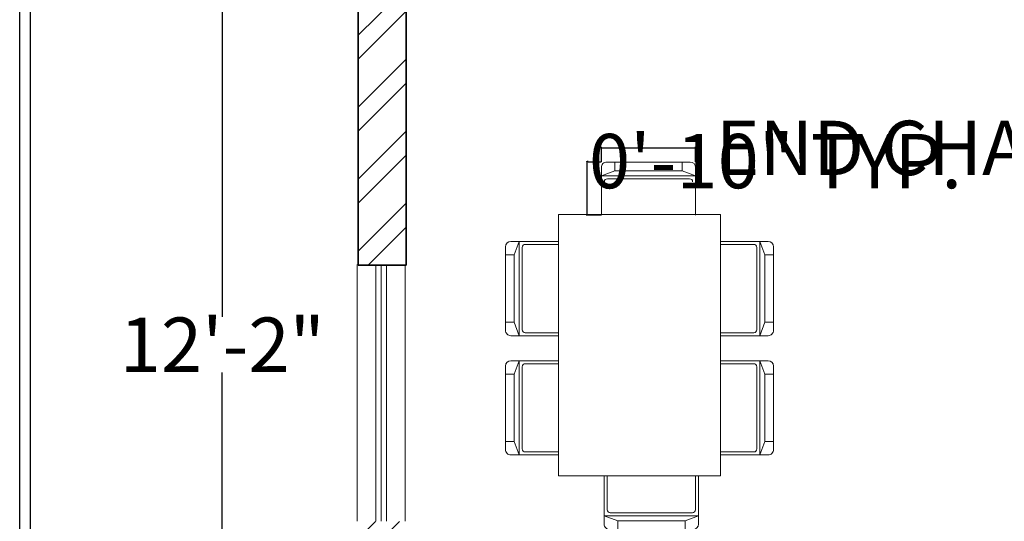
# Model space of a CAD drawing. Units: inches. Extents: x 1812 to 2791, y 2306 to 2959.
# Tile 6 of 8: x 2391 to 2575, y 2655 to 2748. Entities that reach past the tile are written whole.
import ezdxf

# ---------------------------------------------------------------- set-up
doc = ezdxf.new("R2010")
doc.units = ezdxf.units.IN
doc.layers.get('Defpoints').update_dxf_attribs({"lineweight": 50})
for name, color, linetype, lineweight in [('00 FURNITURE', 15, 'Continuous', 15), ('A-ANNO-DIMS', 2, 'Continuous', 18), ('A-ANNO-TTLB', 7, 'Continuous', 25), ('A-WALL-PATT', 8, 'Continuous', 13), ('WALL', 7, 'Continuous', 35), ('WINDOWS', 160, 'Continuous', 18)]:
    doc.layers.add(name, color=color, linetype=linetype, lineweight=lineweight)
doc.styles.get("Standard").update_dxf_attribs({"font": 'arial.ttf'})
doc.dimstyles.get("Standard").update_dxf_attribs({"dimtxt": 10.18, "dimasz": 0.18, "dimexe": 0.18, "dimexo": 0.0625, "dimgap": 0.09, "dimtad": 0, "dimtih": 1, "dimtoh": 1, "dimdec": 0, "dimzin": 0, "dimdsep": 46, "dimlunit": 3, "dimtxsty": 'Standard', "dimcen": 0.09, "dimadec": 0, "dimazin": 0, "dimtfac": 1, "dimtdec": 0, "dimtofl": 0, "dimtmove": 0, "dimatfit": 3, "dimfxl": 1, "dimtolj": 1, "dimtzin": 0, "dimarcsym": 0})

# ---------------------------------------------------------------- blocks, each defined once
blk = doc.blocks.new('CHAIR-DINING')
for p, q in [((-0.0002919860735346, 16.63588649700705), (-0.0003138742495139, 1.018845651208721)), ((9.925763979173098, 17.65493302806589), (1.018765697107482, 17.65494176689844)), ((1.614874244286511, 15.12954713197268), (2.568532326808963, 17.65494024488453)), ((2.568532326808963, 17.65494024488453), (2.568507595072333, -0.0002145154603568)), ((9.925763979173098, 17.09119695253048), (3.692750862651337, 17.09120477086708)), ((1.614874244286511, 15.12954713197268), (1.614856157536451, 2.551355148459151)), ((3.132268951824698, 16.530724333742), (3.132247167491186, 1.124003998030275)), ((1.614856157536451, 2.551355148459151), (2.568507595072333, -0.0002145154603568)), ((3.692727608225141, 0.5635220945378024), (9.925763979173098, 0.5635142763176191)), ((1.018741536737252, -0.0002124476914105), (9.925763979173098, -0.0002237815378976))]:
    blk.add_line(p, q)
blk.add_lwpolyline([(-0.000293857100587, 15.12954925550457), (-0.000311951301228, 2.551357264540456), (1.614856157536451, 2.551355148459151), (1.614874244286511, 15.12954713197268)], close=True)
for centre, radius, start, end in [((1.018764709439892, 16.63588507511031), 1.019056690993971, 89.9999438110219, 179.9999196585658), ((3.692750135055575, 16.53072360987153), 0.5604811800496505, 89.99992486791913, 179.9999248879294), ((1.018742821263913, 1.018844240487851), 1.019056690993971, 179.9999201921744, 269.9999275359618), ((3.692728335820902, 1.124003270434513), 0.5604811800496505, 179.9999248879294, 269.9999248679191)]:
    blk.add_arc(centre, radius, start, end)
blk = doc.blocks.new('CHAIR-DINING-END')
for p, q in [((16.63624727438082, 9.925777952737917), (1.019206428582492, 9.925799840913896)), ((0.0001483296823608, 8.9067444296943), (0.0001369958358737, -0.0002780127415463)), ((2.551715925832922, 8.3106298088951), (0.0001462619134145, 7.356978371592049)), ((15.12990790946287, 8.31061172214504), (2.551715925832922, 8.3106298088951)), ((15.12990790946287, 8.31061172214504), (17.6553010222583, 7.356953639622588)), ((17.65529380532325, -0.0002780127415463), (17.65530254427222, 8.9067202695569)), ((17.6553010222583, 7.356953639622588), (0.0001462619134145, 7.356978371592049)), ((16.53108511111577, 6.793217014839683), (1.124364775520461, 6.793238799173195))]:
    blk.add_line(p, q)
blk.add_lwpolyline([(15.12991003287834, 9.92577982376497), (2.551718041914227, 9.92579791773278), (2.551715925832922, 8.3106298088951), (15.12990790946287, 8.31061172214504)], close=True)
for centre, radius, start, end in [((1.019205017861622, 8.906743145400469), 1.019056690993971, 89.99992015882385, 179.9999275359617), ((16.63624585248408, 8.90672125699166), 1.019056690993971, 359.9999438110219, 89.99991962521533), ((1.124364047808285, 6.232757630610649), 0.5604811800496505, 89.99992490793976, 179.9999248679191), ((16.5310843872453, 6.232735831608806), 0.5604811800496505, 359.9999248679191, 89.99992490793976)]:
    blk.add_arc(centre, radius, start, end)
blk = doc.blocks.new('TABLE-DINING-RECT')
for p, q in [((30.34839303535387, 48.92733218540207), (-0.0002364942340591, 48.92732934110473)), ((-0.0002326415853986, 48.92732934110473), (-0.0002280560938743, 0.0001748373420014)), ((30.34839189378522, 48.92733218540207), (30.34839647927674, 0.0001776816393431)), ((30.34839647927674, 0.0001776816393431), (-0.0002280560934196, 0.0001748373420014))]:
    blk.add_line(p, q)
blk = doc.blocks.new('WINDOW-48x9')
for p, q in [((-0.0002644799014888, 47.99951726123345), (-0.0002644799014888, -0.00048273876655)), ((3.499735520098511, -0.00048273876655), (3.499735520098511, 47.99951726123345)), ((4.499735520098511, -0.00048273876655), (4.499735520098511, 47.99951726123345)), ((5.499735520098511, -0.00048273876655), (5.499735520098511, 47.99951726123345)), ((8.999735520098511, -0.00048273876655), (8.999735520098511, 47.99951726123345))]:
    blk.add_line(p, q)
blk = doc.blocks.new('SHEET-FRAME-RESIDENCE')
blk.add_lwpolyline([(0.000131823559741, 632.8005012919775), (378.7609620870107, 632.8005012919775), (378.7609620870107, 0.0003856501880364), (0.000131823559741, 0.0003856501880364)], close=True)
blk.add_lwpolyline([(2.00013182355974, 71.32450104412055), (2.00013182355974, 630.8005012919775), (376.7609620870107, 630.8005012919775), (376.7609620870107, 71.32450104412055)])
blk = doc.blocks.new('*D64')
at = {"layer": 'A-ANNO-DIMS', "color": 0, "lineweight": -2, "transparency": 16777216}
for p, q in [((2499.736887761388, 2721.901978502181), (2499.736887761388, 2724.667753417118)), ((2499.916887761388, 2724.487753417118), (2517.212053860968, 2724.487753417118)), ((2517.392053860968, 2721.901978502181), (2517.392053860968, 2724.667753417118)), ((2517.392053860968, 2724.487753417118), (2517.572053860968, 2724.487753417118))]:
    blk.add_line(p, q, dxfattribs=at)
at = {"layer": 'A-ANNO-DIMS', "color": 0, "transparency": 16777216}
for points in [[(2499.916887761388, 2724.517753417118), (2499.916887761388, 2724.457753417118), (2499.736887761388, 2724.487753417118)], [(2517.212053860968, 2724.517753417118), (2517.212053860968, 2724.457753417118), (2517.392053860968, 2724.487753417118)]]:
    blk.add_solid(points, dxfattribs=at)
at = {"layer": 'Defpoints', "color": 0, "transparency": 16777216}
for p in [(2517.392053860968, 2724.487753417118), (2499.736887761388, 2721.839478502181), (2517.392053860968, 2721.839478502181)]:
    blk.add_point(p, dxfattribs=at)
at = {"layer": 'A-ANNO-DIMS', "color": 0, "transparency": 16777216, "insert": (2601.369291241595, 2724.487753417118), "char_height": 10.18, "attachment_point": 5}
blk.add_mtext('\\A1;END CHAIR 1\'-5 1/2" TYP.', dxfattribs=at)
blk = doc.blocks.new('*D65')
at = {"layer": 'A-ANNO-DIMS', "color": 0, "lineweight": -2, "transparency": 16777216}
for p, q in [((2499.674387761389, 2721.839478502182), (2496.908612846453, 2721.839478502182)), ((2497.088612846453, 2721.839478502182), (2497.088612846453, 2722.019478502182)), ((2497.088612846453, 2722.019478502182), (2497.268612846453, 2722.019478502182)), ((2497.088612846453, 2712.093400276427), (2497.088612846453, 2721.659478502183)), ((2499.674387761389, 2711.913400276428), (2496.908612846453, 2711.913400276428))]:
    blk.add_line(p, q, dxfattribs=at)
at = {"layer": 'A-ANNO-DIMS', "color": 0, "transparency": 16777216}
for points in [[(2497.058612846453, 2721.659478502183), (2497.118612846453, 2721.659478502183), (2497.088612846453, 2721.839478502182)], [(2497.058612846453, 2712.093400276427), (2497.118612846453, 2712.093400276427), (2497.088612846453, 2711.913400276428)]]:
    blk.add_solid(points, dxfattribs=at)
at = {"layer": 'Defpoints', "color": 0, "transparency": 16777216}
for p in [(2497.088612846453, 2721.839478502182), (2499.736887761389, 2721.839478502182), (2499.736887761389, 2711.913400276428)]:
    blk.add_point(p, dxfattribs=at)
at = {"layer": 'A-ANNO-DIMS', "color": 0, "transparency": 16777216, "insert": (2532.33934272367, 2722.019478502181), "char_height": 10.18, "attachment_point": 5}
blk.add_mtext('\\A1;0\'-10" TYP.', dxfattribs=at)
blk = doc.blocks.new('*D73')
at = {"layer": 'A-ANNO-DIMS', "color": 0, "lineweight": -2, "transparency": 16777216}
for p, q in [((2454.218562000001, 2760.694666000001), (2428.586486000002, 2760.694666000001)), ((2428.766486000002, 2760.514666000001), (2428.766486000002, 2692.848797196454)), ((2428.766486000002, 2614.781264000001), (2428.766486000002, 2682.447132803548)), ((2454.176191000001, 2614.601264000001), (2428.586486000002, 2614.601264000001))]:
    blk.add_line(p, q, dxfattribs=at)
at = {"layer": 'A-ANNO-DIMS', "color": 0, "transparency": 16777216}
for points in [[(2428.736486000002, 2760.514666000001), (2428.796486000002, 2760.514666000001), (2428.766486000002, 2760.694666000001)], [(2428.736486000002, 2614.781264000001), (2428.796486000002, 2614.781264000001), (2428.766486000002, 2614.601264000001)]]:
    blk.add_solid(points, dxfattribs=at)
at = {"layer": 'Defpoints', "color": 0, "transparency": 16777216}
for p in [(2428.766486000002, 2760.694666000001), (2454.281062000001, 2760.694666000001), (2454.238691000001, 2614.601264000001)]:
    blk.add_point(p, dxfattribs=at)
at = {"layer": 'A-ANNO-DIMS', "color": 0, "transparency": 16777216, "insert": (2428.766486000002, 2687.647965), "char_height": 10.18, "attachment_point": 5}
blk.add_mtext('\\A1;12\'-2"', dxfattribs=at)

msp = doc.modelspace()

# ---------------------------------------------------------------- hatches: boundary and pattern name
at = {"layer": 'A-WALL-PATT'}
h = msp.add_hatch(dxfattribs=at)
h.set_pattern_fill('ANSI32', color=256)
h.set_pattern_definition([(45, (563.8057507655523, 20.01067828916757), (-6.735192090801865, 6.735192090801866), []), (45, (568.2958807655523, 20.01067828916757), (-6.735192090801865, 6.735192090801866), [])])
h.paths.add_polyline_path([(2694.192292649419, 2437.613622010101), (2683.499516441466, 2437.6136220101), (2683.499516441466, 2788.569354872347), (2685.192292649419, 2788.569354872347), (2685.192292649419, 2821.63505754476), (2685.125860943268, 2869.374403893766), (2685.125860943268, 2821.63505754476), (2694.192292649419, 2821.63505754476)])
h.paths.add_polyline_path([(2587.192292649419, 2446.613622010096), (2463.19229264942, 2446.613622010089), (2463.19229264942, 2473.613622010101), (2515.608214234135, 2473.613622010101), (2515.608214234135, 2477.6136220101), (2463.19229264942, 2477.6136220101), (2463.19229264942, 2610.6136220101), (2523.737487215154, 2610.613622010101), (2523.737487215154, 2614.613622010101), (2463.19229264942, 2614.6136220101), (2463.19229264942, 2654.536135698824), (2454.192292649419, 2654.536135698824), (2454.192292649419, 2437.613622010101), (2587.192292649419, 2437.613622010101)])
h.paths.add_polyline_path([(2683.499516441466, 2446.6136220101), (2676.19229264942, 2446.6136220101), (2676.192292649419, 2437.6136220101), (2683.499516441466, 2437.613622010101)])
h.paths.add_polyline_path([(2463.192292649419, 2760.6136220101), (2505.192292649419, 2760.6136220101), (2505.192292649419, 2764.6136220101), (2463.192292649419, 2764.6136220101), (2463.192292649419, 2792.952050683902), (2454.192292649419, 2792.952050683902), (2454.192292649419, 2702.536135698824), (2463.016486285651, 2702.536135698824), (2463.016486285651, 2702.649195550402)])
h.paths.add_polyline_path([(2539.192292649419, 2858.613622010101), (2463.192292649419, 2858.6136220101), (2463.192292649419, 2876.345134993912), (2454.192292649419, 2876.345134993912), (2454.19229264942, 2816.957881357627), (2463.192292649419, 2816.957881357627), (2463.192292649419, 2854.6136220101), (2535.192292649419, 2854.613622010101), (2535.192292649419, 2760.6136220101), (2539.192292649419, 2760.6136220101)])
h.paths.add_polyline_path([(2683.499516441466, 2917.613622010101), (2454.192292649419, 2917.613622010101), (2454.192292649419, 2900.372408669677), (2463.192292649419, 2900.372408669677), (2463.192292649419, 2908.6136220101), (2683.499516441466, 2908.613622010101)])
h.paths.add_polyline_path([(2694.192292649419, 2917.613622010101), (2683.499516441466, 2917.613622010101), (2683.499516441466, 2908.613622010101), (2685.192292649419, 2908.613622010101), (2685.192292649419, 2869.63505754476), (2694.192292649419, 2869.63505754476)])

# ---------------------------------------------------------------- linework, layer by layer
at = {"layer": 'WALL'}
for p, q in [((2454.192292649419, 2702.536135698824), (2454.192292649419, 2792.952050683902)), ((2463.19229264942, 2702.536135698824), (2463.192292649419, 2760.6136220101)), ((2454.192292649419, 2702.536135698824), (2463.19229264942, 2702.536135698824))]:
    msp.add_line(p, q, dxfattribs=at)

# ---------------------------------------------------------------- block references
at = {"layer": '00 FURNITURE'}
for name, p in [('CHAIR-DINING-END', (2499.736750765552, 2711.913678289168)), ('CHAIR-DINING', (2481.781750765554, 2689.334678289168)), ('CHAIR-DINING', (2481.781750765532, 2667.005486838955))]:
    msp.add_blockref(name, p, dxfattribs=at)
at = {"layer": '00 FURNITURE', "rotation": 179.9999947369858}
msp.add_blockref('TABLE-DINING-RECT', (2522.055916218236, 2712.020183889784), dxfattribs=at)
at = {"layer": '00 FURNITURE', "extrusion": (0, 0, -1), "zscale": -1}
for p in [(-2531.981908250809, 2689.334678290429), (-2531.981908253542, 2667.005486838922)]:
    msp.add_blockref('CHAIR-DINING', p, dxfattribs=at)
at = {"layer": '00 FURNITURE', "extrusion": (0, 0, -1), "zscale": -1, "rotation": 90.00000000029095}
msp.add_blockref('CHAIR-DINING', (-2500.272413257816, 2653.056076331386), dxfattribs=at)
at = {"layer": 'A-ANNO-TTLB'}
msp.add_blockref('SHEET-FRAME-RESIDENCE', (2390.832750765552, 2326.134678289167), dxfattribs=at)
at = {"layer": 'WINDOWS'}
msp.add_blockref('WINDOW-48x9', (2454.016750765553, 2654.649678289168), dxfattribs=at)

# ---------------------------------------------------------------- dimensions: what is measured, and where the dimension line sits
at = {"layer": 'A-ANNO-DIMS'}
dim = msp.add_linear_dim(base=(2517.392053860968, 2724.487753417118), p1=(2499.736887761388, 2721.839478502181), p2=(2517.392053860968, 2721.839478502181), text='END CHAIR <> TYP.', dimstyle='Standard', override={"dimdec": 1, "dimlfac": 1, "dimrnd": 0, "dimzin": 1, "dimdsep": 46, "dimlunit": 4, "dimfrac": 2}, dxfattribs=at)
dim.commit()
dim.dimension.update_dxf_attribs({"geometry": '*D64', "text_midpoint": (2601.369291241595, 2724.487753417118)})
dim = msp.add_linear_dim(base=(2428.766486000002, 2760.694666000001), p1=(2454.238691, 2614.601264), p2=(2454.281062, 2760.694666), angle=90, dimstyle='Standard', override={"dimdec": 1, "dimlfac": 1, "dimrnd": 0, "dimzin": 1, "dimdsep": 46, "dimlunit": 4, "dimfrac": 2}, dxfattribs=at)
dim.commit()
dim.dimension.update_dxf_attribs({"geometry": '*D73', "text_midpoint": (2428.766486000002, 2687.647965)})
dim = msp.add_linear_dim(base=(2497.088612846453, 2721.839478502182), p1=(2499.736887761388, 2711.913400276426), p2=(2499.736887761388, 2721.839478502181), angle=90, text='<> TYP.', dimstyle='Standard', override={"dimdec": 1, "dimlfac": 1, "dimrnd": 0, "dimzin": 1, "dimdsep": 46, "dimlunit": 4, "dimfrac": 2}, dxfattribs=at)
dim.commit()
dim.dimension.update_dxf_attribs({"geometry": '*D65', "text_midpoint": (2532.33934272367, 2722.019478502181)})

doc.saveas('drawing.dxf')
